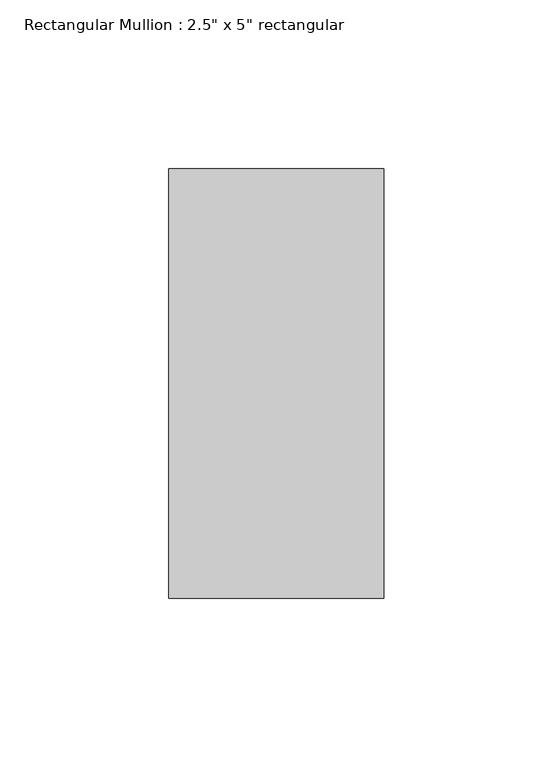
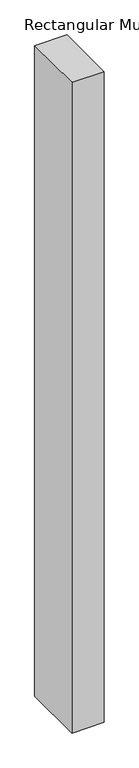
"""IFC4 building model written with IfcOpenShell, lengths in millimetres: member geometry."""

from ifc_helpers import new_model, si_unit, frame, origin, place, context, project, spatial, polyline, outline, extrude, source, transform, mapped, element, save


def member_6ffa5180(model_context):
    return source(origin(), model_context, "Body", "SweptSolid", [
        extrude(outline(polyline([(0.0, 63.5), (0.0, -63.5), (-63.5, -63.5), (-63.5, 63.5), (0.0, 63.5)])), frame((0.0, 0.0, -1359.7734608), z_axis=(0.0, 0.0, 1.0), x_axis=(1.0, 0.0, 0.0)), (0.0, 0.0, 1.0), 1359.7734608),
    ])


if __name__ == "__main__":
    model = new_model("IFC4")
    model_context = context("Model", 3, world=origin())
    ifc_project = project(units=[si_unit("LENGTHUNIT", "METRE", prefix="MILLI")], contexts=[model_context])
    site = spatial("IfcSite", under=ifc_project)
    building = spatial("IfcBuilding", under=site)
    placement = place(None, origin())
    member_shape = member_6ffa5180(model_context)
    element("IfcMember", 1, ObjectType="Rectangular Mullion : 2.5\" x 5\" rectangular", at=placement, inside=building, context=model_context, shape_type="MappedRepresentation", body=[
        mapped(member_shape, transform((0.0, 0.0, 0.0), x_axis=(1.0, 0.0, 0.0), y_axis=(0.0, 1.0, 0.0), z_axis=(0.0, 0.0, 1.0))),
    ])
    save(model, "model.ifc")

# Revit data of these elements
# Type "Rectangular Mullion : 2.5\" x 5\" rectangular"
#   built-in parameter 1007304 = 0.416667 (stored number, unit not read)
#   built-in parameter 1007301 = 0.104167 (stored number, unit not read)
#   built-in parameter 1007300 = 0.104167 (stored number, unit not read)
# Element 1 (IfcMember, "Rectangular Mullion : 2.5\" x 5\" rectangular")
#   Materials on its faces: "Aluminum"
# Materials
#   "Aluminum": class "Metal", colour RGB 247 247 247, transparency 0, Description = "Aluminum 6061", Cost = 0
